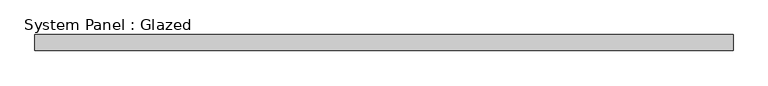
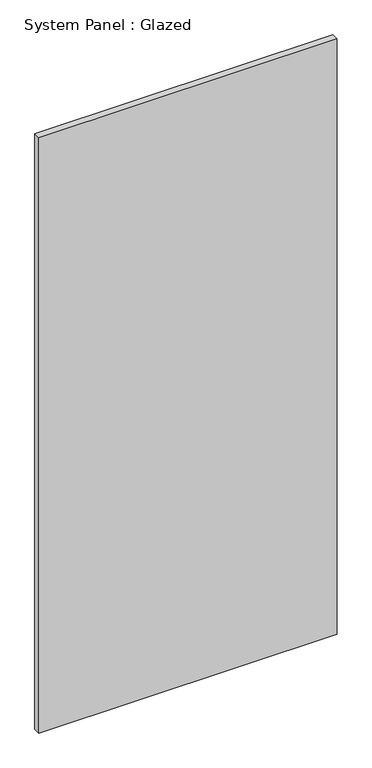
"""IFC4 building model written with IfcOpenShell, lengths in millimetres: plate geometry, System Panel : Glazed."""

from ifc_helpers import new_model, si_unit, origin, origin_with_axes, place, context, project, spatial, polyline, outline, extrude, source, transform, mapped, element, save


def system_panel_glazed_37c910ec(model_context):
    return source(origin(), model_context, "Body", "SweptSolid", [
        extrude(outline(polyline([(555.625, -44.45), (-555.625, -44.45), (-555.625, -19.05), (555.625, -19.05), (555.625, -44.45)])), origin_with_axes(), (0.0, 0.0, 1.0), 2343.15),
    ])


if __name__ == "__main__":
    model = new_model("IFC4")
    model_context = context("Model", 3, world=origin())
    ifc_project = project(units=[si_unit("LENGTHUNIT", "METRE", prefix="MILLI")], contexts=[model_context])
    site = spatial("IfcSite", under=ifc_project)
    building = spatial("IfcBuilding", under=site)
    placement = place(None, origin())
    system_panel_glazed_shape = system_panel_glazed_37c910ec(model_context)
    element("IfcPlate", 1, ObjectType="System Panel : Glazed", at=placement, inside=building, context=model_context, shape_type="MappedRepresentation", body=[
        mapped(system_panel_glazed_shape, transform((0.0, 0.0, 0.0), x_axis=(1.0, 0.0, 0.0), y_axis=(0.0, 1.0, 0.0), z_axis=(0.0, 0.0, 1.0))),
    ])
    save(model, "model.ifc")

# Revit data of these elements
# Type "System Panel : Glazed"
#   Construction Type Id = "GSP4R"
#   Analytic Construction = "1/8 in Pilkington single glazing"
#   Visual Light Transmittance = 0.9
#   Solar Heat Gain Coefficient = 0.86
#   Heat Transfer Coefficient (U) = 1.18115 BTU/(h·ft²·°F)
#   Define Thermal Properties by = 1
# Element 1 (IfcPlate, "System Panel : Glazed")
#   Materials on its faces: "glass panel 223"
# Materials
#   "glass panel 223": class "Generic", colour RGB 120 120 120, transparency 0, Cost = 0
